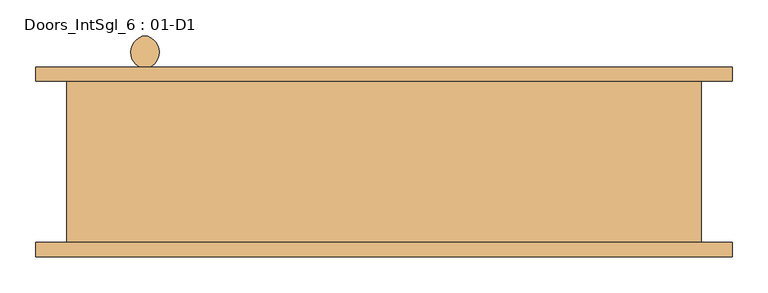
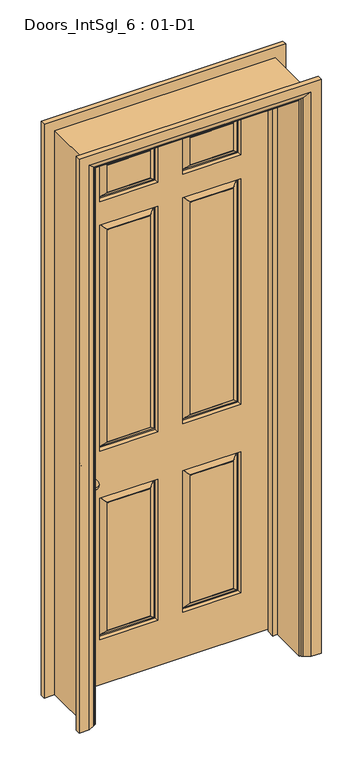
"""IFC4 building model written with IfcOpenShell, lengths in millimetres: door geometry, Doors_IntSgl_6 : 01-D1."""

from ifc_helpers import new_model, si_unit, point, frame, origin, place, context, project, spatial, polyline, circle_curve, ellipse_curve, trimmed, outline, extrude, faceted_brep, source, transform, mapped, element, save
from ifc_brep_helpers import plane_surface, cylinder_surface, revolved_surface, advanced_brep


def doors_intsgl_6_01_d1_adb953bf(model_context):
    return source(origin(), model_context, "Body", "SolidModel", [
        advanced_brep(
        [(-328.0, 55.5, 900.0), (-333.0, 11.062589, 900.0), (-338.0, 55.5, 900.0), (-338.0, 70.5, 900.0), (-328.0, 70.5, 900.0), (-353.0, 74.5, 900.0), (-313.0, 74.5, 900.0), (-353.0, 70.5, 900.0), (-313.0, 70.5, 900.0)],
        [
            (0, 1, circle_curve(frame((-336.1884862, 33.9213505, 900.0), z_axis=(0.0, 0.0, -1.0), x_axis=(0.0, 1.0, 0.0)), 23.0800654)),
            (1, 2, circle_curve(frame((-329.8115138, 33.9213505, 900.0), z_axis=(0.0, 0.0, -1.0), x_axis=(0.0, 1.0, 0.0)), 23.0800654)),
            (2, 0, circle_curve(frame((-333.0, 55.5, 900.0), z_axis=(0.0, -1.0, 0.0), x_axis=(-1.0, 0.0, 0.0)), 5.0)),
            (0, 2, circle_curve(frame((-333.0, 55.5, 900.0), z_axis=(0.0, -1.0, 0.0), x_axis=(-1.0, 0.0, 0.0)), 5.0)),
            (2, 3),
            (3, 4, circle_curve(frame((-333.0, 70.5, 900.0), z_axis=(0.0, -1.0, 0.0), x_axis=(-1.0, 0.0, 0.0)), 5.0)),
            (4, 0),
            (4, 3, circle_curve(frame((-333.0, 70.5, 900.0), z_axis=(0.0, -1.0, 0.0), x_axis=(-1.0, 0.0, 0.0)), 5.0)),
            (5, 6, circle_curve(frame((-333.0, 74.5, 900.0), z_axis=(0.0, 1.0, 0.0), x_axis=(1.0, 0.0, 0.0)), 20.0)),
            (6, 5, circle_curve(frame((-333.0, 74.5, 900.0), z_axis=(0.0, 1.0, 0.0), x_axis=(1.0, 0.0, 0.0)), 20.0)),
            (7, 8, circle_curve(frame((-333.0, 70.5, 900.0), z_axis=(0.0, -1.0, 0.0), x_axis=(1.0, 0.0, 0.0)), 20.0)),
            (8, 7, circle_curve(frame((-333.0, 70.5, 900.0), z_axis=(0.0, -1.0, 0.0), x_axis=(1.0, 0.0, 0.0)), 20.0)),
            (6, 8),
            (7, 5),
        ],
        [
            revolved_surface(trimmed(ellipse_curve(frame((-329.8115138, 33.9213505, 900.0), z_axis=(0.0, 0.0, -1.0), x_axis=(0.0, 1.0, 0.0)), 23.0800654, 23.0800654), [point((-333.0, 11.062589, 900.0))], [point((-338.0, 55.5, 900.0))], True, "CARTESIAN"), (-333.0, 70.5, 900.0), (0.0, 1.0, 0.0)),
            cylinder_surface(frame((-333.0, 70.5, 900.0), z_axis=(0.0, 1.0, 0.0), x_axis=(-1.0, 0.0, 0.0)), 5.0),
            plane_surface(frame((-313.0, 74.5, 900.0), z_axis=(0.0, 1.0, 0.0), x_axis=(0.0, 0.0, 1.0))),
            plane_surface(frame((-313.0, 70.5, 900.0), z_axis=(0.0, -1.0, 0.0), x_axis=(0.0, 0.0, -1.0))),
            cylinder_surface(frame((-333.0, 70.5, 900.0), z_axis=(0.0, 1.0, 0.0), x_axis=(1.0, 0.0, 0.0)), 20.0),
        ],
        [
            (0, [[1, 2, 3]]),
            (0, [[-1, 4, -2]]),
            (1, [[5, 6, 7, -3]]),
            (1, [[-7, 8, -5, -4]]),
            (2, [[9, 10]]),
            (3, [[11, 12], [-8, -6]]),
            (4, [[13, -11, 14, -10]]),
            (4, [[-14, -12, -13, -9]]),
        ],
    ),
        advanced_brep(
        [(-328.0, 131.5, 900.0), (-338.0, 131.5, 900.0), (-333.0, 175.937411, 900.0), (-328.0, 116.5, 900.0), (-338.0, 116.5, 900.0), (-353.0, 112.5, 900.0), (-313.0, 112.5, 900.0), (-353.0, 116.5, 900.0), (-313.0, 116.5, 900.0)],
        [
            (0, 1, circle_curve(frame((-333.0, 131.5, 900.0), z_axis=(0.0, 1.0, 0.0), x_axis=(-1.0, 0.0, 0.0)), 5.0)),
            (1, 2, circle_curve(frame((-329.8115138, 153.0786495, 900.0), z_axis=(0.0, 0.0, -1.0), x_axis=(0.0, -1.0, 0.0)), 23.0800654)),
            (2, 0, circle_curve(frame((-336.1884862, 153.0786495, 900.0), z_axis=(0.0, 0.0, -1.0), x_axis=(0.0, -1.0, 0.0)), 23.0800654)),
            (1, 0, circle_curve(frame((-333.0, 131.5, 900.0), z_axis=(0.0, 1.0, 0.0), x_axis=(-1.0, 0.0, 0.0)), 5.0)),
            (0, 3),
            (3, 4, circle_curve(frame((-333.0, 116.5, 900.0), z_axis=(0.0, 1.0, 0.0), x_axis=(-1.0, 0.0, 0.0)), 5.0)),
            (4, 1),
            (4, 3, circle_curve(frame((-333.0, 116.5, 900.0), z_axis=(0.0, 1.0, 0.0), x_axis=(-1.0, 0.0, 0.0)), 5.0)),
            (5, 6, circle_curve(frame((-333.0, 112.5, 900.0), z_axis=(0.0, -1.0, 0.0), x_axis=(1.0, 0.0, 0.0)), 20.0)),
            (6, 5, circle_curve(frame((-333.0, 112.5, 900.0), z_axis=(0.0, -1.0, 0.0), x_axis=(1.0, 0.0, 0.0)), 20.0)),
            (7, 8, circle_curve(frame((-333.0, 116.5, 900.0), z_axis=(0.0, 1.0, 0.0), x_axis=(1.0, 0.0, 0.0)), 20.0)),
            (8, 7, circle_curve(frame((-333.0, 116.5, 900.0), z_axis=(0.0, 1.0, 0.0), x_axis=(1.0, 0.0, 0.0)), 20.0)),
            (5, 7),
            (8, 6),
        ],
        [
            revolved_surface(trimmed(ellipse_curve(frame((-329.8115138, 153.0786495, 900.0), z_axis=(0.0, 0.0, 1.0), x_axis=(0.0, -1.0, 0.0)), 23.0800654, 23.0800654), [point((-333.0, 175.937411, 900.0))], [point((-338.0, 131.5, 900.0))], True, "CARTESIAN"), (-333.0, 116.5, 900.0), (0.0, -1.0, 0.0)),
            cylinder_surface(frame((-333.0, 116.5, 900.0), z_axis=(0.0, -1.0, 0.0), x_axis=(-1.0, 0.0, 0.0)), 5.0),
            plane_surface(frame((-313.0, 112.5, 900.0), z_axis=(0.0, -1.0, 0.0), x_axis=(0.0, 0.0, 1.0))),
            plane_surface(frame((-313.0, 116.5, 900.0), z_axis=(0.0, 1.0, 0.0), x_axis=(0.0, 0.0, -1.0))),
            cylinder_surface(frame((-333.0, 116.5, 900.0), z_axis=(0.0, -1.0, 0.0), x_axis=(1.0, 0.0, 0.0)), 20.0),
        ],
        [
            (0, [[1, 2, 3]]),
            (0, [[-2, 4, -3]]),
            (1, [[-1, 5, 6, 7]]),
            (1, [[-4, -7, 8, -5]]),
            (2, [[9, 10]]),
            (3, [[11, 12], [-6, -8]]),
            (4, [[-9, 13, -12, 14]]),
            (4, [[-10, -14, -11, -13]]),
        ],
    ),
        faceted_brep([(-408.0, 74.5, 2358.0), (-408.0, 74.5, 8.0), (408.0, 74.5, 8.0), (408.0, 74.5, 2358.0), (-50.0, 74.5, 800.0), (-50.0, 74.5, 200.0), (-283.0, 74.5, 200.0), (-283.0, 74.5, 800.0), (283.0, 74.5, 800.0), (283.0, 74.5, 200.0), (50.0, 74.5, 200.0), (50.0, 74.5, 800.0), (-50.0, 74.5, 1958.0), (-50.0, 74.5, 1000.0), (-283.0, 74.5, 1000.0), (-283.0, 74.5, 1958.0), (283.0, 74.5, 1958.0), (283.0, 74.5, 1000.0), (50.0, 74.5, 1000.0), (50.0, 74.5, 1958.0), (-50.0, 74.5, 2233.0), (-50.0, 74.5, 2058.0), (-283.0, 74.5, 2058.0), (-283.0, 74.5, 2233.0), (283.0, 74.5, 2233.0), (283.0, 74.5, 2058.0), (50.0, 74.5, 2058.0), (50.0, 74.5, 2233.0), (-80.0, 74.5, 230.0), (-80.0, 74.5, 770.0), (-253.0, 74.5, 770.0), (-253.0, 74.5, 230.0), (253.0, 74.5, 230.0), (253.0, 74.5, 770.0), (80.0, 74.5, 770.0), (80.0, 74.5, 230.0), (-80.0, 74.5, 1030.0), (-80.0, 74.5, 1928.0), (-253.0, 74.5, 1928.0), (-253.0, 74.5, 1030.0), (253.0, 74.5, 1030.0), (253.0, 74.5, 1928.0), (80.0, 74.5, 1928.0), (80.0, 74.5, 1030.0), (-80.0, 74.5, 2088.0), (-80.0, 74.5, 2203.0), (-253.0, 74.5, 2203.0), (-253.0, 74.5, 2088.0), (253.0, 74.5, 2088.0), (253.0, 74.5, 2203.0), (80.0, 74.5, 2203.0), (80.0, 74.5, 2088.0), (-408.0, 112.5, 2358.0), (408.0, 112.5, 2358.0), (408.0, 112.5, 8.0), (-408.0, 112.5, 8.0), (50.0, 112.5, 800.0), (50.0, 112.5, 200.0), (283.0, 112.5, 200.0), (283.0, 112.5, 800.0), (-283.0, 112.5, 800.0), (-283.0, 112.5, 200.0), (-50.0, 112.5, 200.0), (-50.0, 112.5, 800.0), (50.0, 112.5, 1958.0), (50.0, 112.5, 1000.0), (283.0, 112.5, 1000.0), (283.0, 112.5, 1958.0), (-283.0, 112.5, 1958.0), (-283.0, 112.5, 1000.0), (-50.0, 112.5, 1000.0), (-50.0, 112.5, 1958.0), (50.0, 112.5, 2233.0), (50.0, 112.5, 2058.0), (283.0, 112.5, 2058.0), (283.0, 112.5, 2233.0), (-283.0, 112.5, 2233.0), (-283.0, 112.5, 2058.0), (-50.0, 112.5, 2058.0), (-50.0, 112.5, 2233.0), (80.0, 112.5, 230.0), (80.0, 112.5, 770.0), (253.0, 112.5, 770.0), (253.0, 112.5, 230.0), (-253.0, 112.5, 230.0), (-253.0, 112.5, 770.0), (-80.0, 112.5, 770.0), (-80.0, 112.5, 230.0), (80.0, 112.5, 1030.0), (80.0, 112.5, 1928.0), (253.0, 112.5, 1928.0), (253.0, 112.5, 1030.0), (-253.0, 112.5, 1030.0), (-253.0, 112.5, 1928.0), (-80.0, 112.5, 1928.0), (-80.0, 112.5, 1030.0), (80.0, 112.5, 2088.0), (80.0, 112.5, 2203.0), (253.0, 112.5, 2203.0), (253.0, 112.5, 2088.0), (-253.0, 112.5, 2088.0), (-253.0, 112.5, 2203.0), (-80.0, 112.5, 2203.0), (-80.0, 112.5, 2088.0), (80.0, 111.5, 230.0), (80.0, 111.5, 770.0), (58.0, 97.5, 208.0), (58.0, 97.5, 792.0), (78.0, 111.5, 772.0), (78.0, 111.5, 228.0), (53.0, 97.5, 797.0), (53.0, 97.5, 203.0), (253.0, 111.5, 770.0), (275.0, 97.5, 792.0), (255.0, 111.5, 772.0), (280.0, 97.5, 797.0), (253.0, 111.5, 230.0), (275.0, 97.5, 208.0), (255.0, 111.5, 228.0), (280.0, 97.5, 203.0), (-253.0, 111.5, 230.0), (-253.0, 111.5, 770.0), (-275.0, 97.5, 208.0), (-275.0, 97.5, 792.0), (-255.0, 111.5, 772.0), (-255.0, 111.5, 228.0), (-280.0, 97.5, 797.0), (-280.0, 97.5, 203.0), (-80.0, 111.5, 770.0), (-58.0, 97.5, 792.0), (-78.0, 111.5, 772.0), (-53.0, 97.5, 797.0), (-80.0, 111.5, 230.0), (-58.0, 97.5, 208.0), (-78.0, 111.5, 228.0), (-53.0, 97.5, 203.0), (80.0, 111.5, 1030.0), (80.0, 111.5, 1928.0), (58.0, 97.5, 1008.0), (58.0, 97.5, 1950.0), (78.0, 111.5, 1930.0), (78.0, 111.5, 1028.0), (53.0, 97.5, 1955.0), (53.0, 97.5, 1003.0), (253.0, 111.5, 1928.0), (275.0, 97.5, 1950.0), (255.0, 111.5, 1930.0), (280.0, 97.5, 1955.0), (253.0, 111.5, 1030.0), (275.0, 97.5, 1008.0), (255.0, 111.5, 1028.0), (280.0, 97.5, 1003.0), (-253.0, 111.5, 1030.0), (-253.0, 111.5, 1928.0), (-275.0, 97.5, 1008.0), (-275.0, 97.5, 1950.0), (-255.0, 111.5, 1930.0), (-255.0, 111.5, 1028.0), (-280.0, 97.5, 1955.0), (-280.0, 97.5, 1003.0), (-80.0, 111.5, 1928.0), (-58.0, 97.5, 1950.0), (-78.0, 111.5, 1930.0), (-53.0, 97.5, 1955.0), (-80.0, 111.5, 1030.0), (-58.0, 97.5, 1008.0), (-78.0, 111.5, 1028.0), (-53.0, 97.5, 1003.0), (80.0, 111.5, 2088.0), (80.0, 111.5, 2203.0), (58.0, 97.5, 2066.0), (58.0, 97.5, 2225.0), (78.0, 111.5, 2205.0), (78.0, 111.5, 2086.0), (53.0, 97.5, 2230.0), (53.0, 97.5, 2061.0), (253.0, 111.5, 2203.0), (275.0, 97.5, 2225.0), (255.0, 111.5, 2205.0), (280.0, 97.5, 2230.0), (253.0, 111.5, 2088.0), (275.0, 97.5, 2066.0), (255.0, 111.5, 2086.0), (280.0, 97.5, 2061.0), (-253.0, 111.5, 2088.0), (-253.0, 111.5, 2203.0), (-275.0, 97.5, 2066.0), (-275.0, 97.5, 2225.0), (-255.0, 111.5, 2205.0), (-255.0, 111.5, 2086.0), (-280.0, 97.5, 2230.0), (-280.0, 97.5, 2061.0), (-80.0, 111.5, 2203.0), (-58.0, 97.5, 2225.0), (-78.0, 111.5, 2205.0), (-53.0, 97.5, 2230.0), (-80.0, 111.5, 2088.0), (-58.0, 97.5, 2066.0), (-78.0, 111.5, 2086.0), (-53.0, 97.5, 2061.0), (-80.0, 75.5, 230.0), (-80.0, 75.5, 770.0), (-58.0, 89.5, 208.0), (-58.0, 89.5, 792.0), (-78.0, 75.5, 772.0), (-78.0, 75.5, 228.0), (-53.0, 89.5, 797.0), (-53.0, 89.5, 203.0), (-253.0, 75.5, 770.0), (-275.0, 89.5, 792.0), (-255.0, 75.5, 772.0), (-280.0, 89.5, 797.0), (-253.0, 75.5, 230.0), (-275.0, 89.5, 208.0), (-255.0, 75.5, 228.0), (-280.0, 89.5, 203.0), (253.0, 75.5, 230.0), (253.0, 75.5, 770.0), (275.0, 89.5, 208.0), (275.0, 89.5, 792.0), (255.0, 75.5, 772.0), (255.0, 75.5, 228.0), (280.0, 89.5, 797.0), (280.0, 89.5, 203.0), (80.0, 75.5, 770.0), (58.0, 89.5, 792.0), (78.0, 75.5, 772.0), (53.0, 89.5, 797.0), (80.0, 75.5, 230.0), (58.0, 89.5, 208.0), (78.0, 75.5, 228.0), (53.0, 89.5, 203.0), (-80.0, 75.5, 1030.0), (-80.0, 75.5, 1928.0), (-58.0, 89.5, 1008.0), (-58.0, 89.5, 1950.0), (-78.0, 75.5, 1930.0), (-78.0, 75.5, 1028.0), (-53.0, 89.5, 1955.0), (-53.0, 89.5, 1003.0), (-253.0, 75.5, 1928.0), (-275.0, 89.5, 1950.0), (-255.0, 75.5, 1930.0), (-280.0, 89.5, 1955.0), (-253.0, 75.5, 1030.0), (-275.0, 89.5, 1008.0), (-255.0, 75.5, 1028.0), (-280.0, 89.5, 1003.0), (253.0, 75.5, 1030.0), (253.0, 75.5, 1928.0), (275.0, 89.5, 1008.0), (275.0, 89.5, 1950.0), (255.0, 75.5, 1930.0), (255.0, 75.5, 1028.0), (280.0, 89.5, 1955.0), (280.0, 89.5, 1003.0), (80.0, 75.5, 1928.0), (58.0, 89.5, 1950.0), (78.0, 75.5, 1930.0), (53.0, 89.5, 1955.0), (80.0, 75.5, 1030.0), (58.0, 89.5, 1008.0), (78.0, 75.5, 1028.0), (53.0, 89.5, 1003.0), (-80.0, 75.5, 2088.0), (-80.0, 75.5, 2203.0), (-58.0, 89.5, 2066.0), (-58.0, 89.5, 2225.0), (-78.0, 75.5, 2205.0), (-78.0, 75.5, 2086.0), (-53.0, 89.5, 2230.0), (-53.0, 89.5, 2061.0), (-253.0, 75.5, 2203.0), (-275.0, 89.5, 2225.0), (-255.0, 75.5, 2205.0), (-280.0, 89.5, 2230.0), (-253.0, 75.5, 2088.0), (-275.0, 89.5, 2066.0), (-255.0, 75.5, 2086.0), (-280.0, 89.5, 2061.0), (253.0, 75.5, 2088.0), (253.0, 75.5, 2203.0), (275.0, 89.5, 2066.0), (275.0, 89.5, 2225.0), (255.0, 75.5, 2205.0), (255.0, 75.5, 2086.0), (280.0, 89.5, 2230.0), (280.0, 89.5, 2061.0), (80.0, 75.5, 2203.0), (58.0, 89.5, 2225.0), (78.0, 75.5, 2205.0), (53.0, 89.5, 2230.0), (80.0, 75.5, 2088.0), (58.0, 89.5, 2066.0), (78.0, 75.5, 2086.0), (53.0, 89.5, 2061.0)], [[[0, 1, 2, 3], [4, 5, 6, 7], [8, 9, 10, 11], [12, 13, 14, 15], [16, 17, 18, 19], [20, 21, 22, 23], [24, 25, 26, 27]], [[28, 29, 30, 31]], [[32, 33, 34, 35]], [[36, 37, 38, 39]], [[40, 41, 42, 43]], [[44, 45, 46, 47]], [[48, 49, 50, 51]], [[52, 53, 54, 55], [56, 57, 58, 59], [60, 61, 62, 63], [64, 65, 66, 67], [68, 69, 70, 71], [72, 73, 74, 75], [76, 77, 78, 79]], [[80, 81, 82, 83]], [[84, 85, 86, 87]], [[88, 89, 90, 91]], [[92, 93, 94, 95]], [[96, 97, 98, 99]], [[100, 101, 102, 103]], [[1, 0, 52, 55]], [[2, 1, 55, 54]], [[3, 2, 54, 53]], [[0, 3, 53, 52]], [[104, 105, 81, 80]], [[106, 107, 108, 109]], [[56, 110, 111, 57]], [[81, 105, 112, 82]], [[108, 107, 113, 114]], [[110, 56, 59, 115]], [[82, 112, 116, 83]], [[114, 113, 117, 118]], [[115, 59, 58, 119]], [[104, 80, 83, 116]], [[109, 108, 114, 118], [105, 104, 116, 112]], [[106, 109, 118, 117]], [[111, 110, 115, 119], [107, 106, 117, 113]], [[57, 111, 119, 58]], [[120, 121, 85, 84]], [[122, 123, 124, 125]], [[60, 126, 127, 61]], [[85, 121, 128, 86]], [[124, 123, 129, 130]], [[126, 60, 63, 131]], [[86, 128, 132, 87]], [[130, 129, 133, 134]], [[131, 63, 62, 135]], [[120, 84, 87, 132]], [[125, 124, 130, 134], [121, 120, 132, 128]], [[122, 125, 134, 133]], [[127, 126, 131, 135], [123, 122, 133, 129]], [[61, 127, 135, 62]], [[136, 137, 89, 88]], [[138, 139, 140, 141]], [[64, 142, 143, 65]], [[89, 137, 144, 90]], [[140, 139, 145, 146]], [[142, 64, 67, 147]], [[90, 144, 148, 91]], [[146, 145, 149, 150]], [[147, 67, 66, 151]], [[136, 88, 91, 148]], [[141, 140, 146, 150], [137, 136, 148, 144]], [[138, 141, 150, 149]], [[143, 142, 147, 151], [139, 138, 149, 145]], [[65, 143, 151, 66]], [[152, 153, 93, 92]], [[154, 155, 156, 157]], [[68, 158, 159, 69]], [[93, 153, 160, 94]], [[156, 155, 161, 162]], [[158, 68, 71, 163]], [[94, 160, 164, 95]], [[162, 161, 165, 166]], [[163, 71, 70, 167]], [[152, 92, 95, 164]], [[157, 156, 162, 166], [153, 152, 164, 160]], [[154, 157, 166, 165]], [[159, 158, 163, 167], [155, 154, 165, 161]], [[69, 159, 167, 70]], [[168, 169, 97, 96]], [[170, 171, 172, 173]], [[72, 174, 175, 73]], [[97, 169, 176, 98]], [[172, 171, 177, 178]], [[174, 72, 75, 179]], [[98, 176, 180, 99]], [[178, 177, 181, 182]], [[179, 75, 74, 183]], [[168, 96, 99, 180]], [[173, 172, 178, 182], [169, 168, 180, 176]], [[170, 173, 182, 181]], [[175, 174, 179, 183], [171, 170, 181, 177]], [[73, 175, 183, 74]], [[184, 185, 101, 100]], [[186, 187, 188, 189]], [[76, 190, 191, 77]], [[101, 185, 192, 102]], [[188, 187, 193, 194]], [[190, 76, 79, 195]], [[102, 192, 196, 103]], [[194, 193, 197, 198]], [[195, 79, 78, 199]], [[184, 100, 103, 196]], [[189, 188, 194, 198], [185, 184, 196, 192]], [[186, 189, 198, 197]], [[191, 190, 195, 199], [187, 186, 197, 193]], [[77, 191, 199, 78]], [[200, 201, 29, 28]], [[202, 203, 204, 205]], [[4, 206, 207, 5]], [[29, 201, 208, 30]], [[204, 203, 209, 210]], [[206, 4, 7, 211]], [[30, 208, 212, 31]], [[210, 209, 213, 214]], [[211, 7, 6, 215]], [[200, 28, 31, 212]], [[205, 204, 210, 214], [201, 200, 212, 208]], [[202, 205, 214, 213]], [[207, 206, 211, 215], [203, 202, 213, 209]], [[5, 207, 215, 6]], [[216, 217, 33, 32]], [[218, 219, 220, 221]], [[8, 222, 223, 9]], [[33, 217, 224, 34]], [[220, 219, 225, 226]], [[222, 8, 11, 227]], [[34, 224, 228, 35]], [[226, 225, 229, 230]], [[227, 11, 10, 231]], [[216, 32, 35, 228]], [[221, 220, 226, 230], [217, 216, 228, 224]], [[218, 221, 230, 229]], [[223, 222, 227, 231], [219, 218, 229, 225]], [[9, 223, 231, 10]], [[232, 233, 37, 36]], [[234, 235, 236, 237]], [[12, 238, 239, 13]], [[37, 233, 240, 38]], [[236, 235, 241, 242]], [[238, 12, 15, 243]], [[38, 240, 244, 39]], [[242, 241, 245, 246]], [[243, 15, 14, 247]], [[232, 36, 39, 244]], [[237, 236, 242, 246], [233, 232, 244, 240]], [[234, 237, 246, 245]], [[239, 238, 243, 247], [235, 234, 245, 241]], [[13, 239, 247, 14]], [[248, 249, 41, 40]], [[250, 251, 252, 253]], [[16, 254, 255, 17]], [[41, 249, 256, 42]], [[252, 251, 257, 258]], [[254, 16, 19, 259]], [[42, 256, 260, 43]], [[258, 257, 261, 262]], [[259, 19, 18, 263]], [[248, 40, 43, 260]], [[253, 252, 258, 262], [249, 248, 260, 256]], [[250, 253, 262, 261]], [[255, 254, 259, 263], [251, 250, 261, 257]], [[17, 255, 263, 18]], [[264, 265, 45, 44]], [[266, 267, 268, 269]], [[20, 270, 271, 21]], [[45, 265, 272, 46]], [[268, 267, 273, 274]], [[270, 20, 23, 275]], [[46, 272, 276, 47]], [[274, 273, 277, 278]], [[275, 23, 22, 279]], [[264, 44, 47, 276]], [[269, 268, 274, 278], [265, 264, 276, 272]], [[266, 269, 278, 277]], [[271, 270, 275, 279], [267, 266, 277, 273]], [[21, 271, 279, 22]], [[280, 281, 49, 48]], [[282, 283, 284, 285]], [[24, 286, 287, 25]], [[49, 281, 288, 50]], [[284, 283, 289, 290]], [[286, 24, 27, 291]], [[50, 288, 292, 51]], [[290, 289, 293, 294]], [[291, 27, 26, 295]], [[280, 48, 51, 292]], [[285, 284, 290, 294], [281, 280, 292, 288]], [[282, 285, 294, 293]], [[287, 286, 291, 295], [283, 282, 293, 289]], [[25, 287, 295, 26]]]),
        faceted_brep([(-410.0, 112.5, 0.0), (-410.0, -112.5, 0.0), (-442.0, -112.5, 0.0), (-442.0, 112.5, 0.0), (-410.0, 112.5, 2360.0), (-410.0, -112.5, 2360.0), (-442.0, -112.5, 2392.0), (-442.0, 112.5, 2392.0), (410.0, 112.5, 0.0), (442.0, 112.5, 0.0), (442.0, -112.5, 0.0), (410.0, -112.5, 0.0), (410.0, 112.5, 2360.0), (442.0, 112.5, 2392.0), (442.0, -112.5, 2392.0), (410.0, -112.5, 2360.0)], [[[0, 1, 2, 3]], [[1, 0, 4, 5]], [[2, 1, 5, 6]], [[3, 2, 6, 7]], [[0, 3, 7, 4]], [[8, 9, 10, 11]], [[12, 13, 9, 8]], [[13, 14, 10, 9]], [[14, 15, 11, 10]], [[15, 12, 8, 11]], [[5, 4, 12, 15]], [[6, 5, 15, 14]], [[7, 6, 14, 13]], [[4, 7, 13, 12]]]),
        extrude(outline(polyline([(0.0, -410.0), (0.0, -391.0), (2341.0, -391.0), (2341.0, 391.0), (0.0, 391.0), (0.0, 410.0), (2360.0, 410.0), (2360.0, -410.0), (0.0, -410.0)])), frame((0.0, 40.5, 0.0), z_axis=(0.0, 1.0, 0.0), x_axis=(0.0, 0.0, 1.0)), (0.0, 0.0, 1.0), 32.0),
        advanced_brep(
        [(-485.0, -132.5, 0.0), (-485.0, -112.5, 0.0), (-415.0, -112.5, 0.0), (-419.0, -118.5, 0.0), (-445.0, -132.5, 0.0), (-485.0, -132.5, 2435.0), (-485.0, -112.5, 2435.0), (485.0, -112.5, 2435.0), (485.0, -112.5, 0.0), (415.0, -112.5, 0.0), (415.0, -112.5, 2365.0), (-415.0, -112.5, 2365.0), (-419.0, -118.5, 2369.0), (-445.0, -132.5, 2395.0), (445.0, -132.5, 2395.0), (445.0, -132.5, 0.0), (485.0, -132.5, 0.0), (485.0, -132.5, 2435.0), (419.0, -118.5, 0.0), (419.0, -118.5, 2369.0)],
        [
            (0, 1),
            (1, 2),
            (2, 3, circle_curve(frame((-423.0, -111.5, 0.0), z_axis=(0.0, 0.0, -1.0), x_axis=(-1.0, 0.0, 0.0)), 8.0622577)),
            (3, 4),
            (4, 0),
            (0, 5),
            (5, 6),
            (6, 1),
            (6, 7),
            (7, 8),
            (8, 9),
            (9, 10),
            (10, 11),
            (11, 2),
            (11, 12, ellipse_curve(frame((-423.0, -111.5, 2373.0), z_axis=(-0.7071067811865475, 0.0, -0.7071067811865475), x_axis=(0.7071067811865474, 0.0, -0.7071067811865476)), 11.4017543, 8.0622577)),
            (12, 3),
            (12, 13),
            (13, 4),
            (13, 14),
            (14, 15),
            (15, 16),
            (16, 17),
            (17, 5),
            (7, 17),
            (16, 8),
            (15, 18),
            (18, 9, circle_curve(frame((423.0, -111.5, 0.0), z_axis=(0.0, 0.0, -1.0), x_axis=(1.0, 0.0, 0.0)), 8.0622577)),
            (19, 10, ellipse_curve(frame((423.0, -111.5, 2373.0), z_axis=(0.7071067811865475, 0.0, -0.7071067811865475), x_axis=(0.7071067811865474, 0.0, 0.7071067811865476)), 11.4017543, 8.0622577)),
            (18, 19),
            (14, 19),
            (19, 12),
        ],
        [
            plane_surface(frame((-415.0, -112.5, 0.0), z_axis=(0.0, 0.0, -1.0), x_axis=(0.0, -1.0, 0.0))),
            plane_surface(frame((-485.0, -132.5, 0.0), z_axis=(-1.0, 0.0, 0.0), x_axis=(0.0, 0.0, 1.0))),
            plane_surface(frame((-485.0, -112.5, 0.0), z_axis=(0.0, 1.0, 0.0), x_axis=(0.0, 0.0, 1.0))),
            cylinder_surface(frame((-423.0, -111.5, 0.0), z_axis=(0.0, 0.0, -1.0), x_axis=(-1.0, 0.0, 0.0)), 8.0622577),
            plane_surface(frame((-419.0, -118.5, 0.0), z_axis=(0.4740998230350183, -0.8804710999221749, 0.0), x_axis=(0.0, 0.0, 1.0))),
            plane_surface(frame((-445.0, -132.5, 0.0), z_axis=(0.0, -1.0, 0.0), x_axis=(0.0, 0.0, 1.0))),
            plane_surface(frame((485.0, -132.5, 2435.0), z_axis=(1.0, 0.0, 0.0), x_axis=(0.0, 0.0, -1.0))),
            plane_surface(frame((415.0, -112.5, 0.0), z_axis=(0.0, 0.0, -1.0), x_axis=(0.0, -1.0, 0.0))),
            cylinder_surface(frame((423.0, -111.5, 2365.0), z_axis=(0.0, 0.0, 1.0), x_axis=(1.0, 0.0, 0.0)), 8.0622577),
            plane_surface(frame((419.0, -118.5, 2369.0), z_axis=(-0.4740998230350183, -0.8804710999221749, 0.0), x_axis=(0.0, 0.0, -1.0))),
            plane_surface(frame((-485.0, -132.5, 2435.0), z_axis=(0.0, 0.0, 1.0), x_axis=(1.0, 0.0, 0.0))),
            cylinder_surface(frame((-415.0, -111.5, 2373.0), z_axis=(-1.0, 0.0, 0.0), x_axis=(0.0, 0.0, 1.0)), 8.0622577),
            plane_surface(frame((-419.0, -118.5, 2369.0), z_axis=(0.0, -0.8804710999221749, -0.4740998230350183), x_axis=(1.0, 0.0, 0.0))),
        ],
        [
            (0, [[1, 2, 3, 4, 5]]),
            (1, [[-1, 6, 7, 8]]),
            (2, [[-2, -8, 9, 10, 11, 12, 13, 14]]),
            (3, [[-3, -14, 15, 16]]),
            (4, [[-4, -16, 17, 18]]),
            (5, [[-5, -18, 19, 20, 21, 22, 23, -6]]),
            (6, [[24, -22, 25, -10]]),
            (7, [[-21, 26, 27, -11, -25]]),
            (8, [[28, -12, -27, 29]]),
            (9, [[30, -29, -26, -20]]),
            (10, [[-7, -23, -24, -9]]),
            (11, [[-15, -13, -28, 31]]),
            (12, [[-17, -31, -30, -19]]),
        ],
    ),
        advanced_brep(
        [(485.0, 132.5, 0.0), (485.0, 112.5, 0.0), (415.0, 112.5, 0.0), (419.0, 118.5, 0.0), (445.0, 132.5, 0.0), (485.0, 132.5, 2435.0), (485.0, 112.5, 2435.0), (-485.0, 112.5, 2435.0), (-485.0, 112.5, 0.0), (-415.0, 112.5, 0.0), (-415.0, 112.5, 2365.0), (415.0, 112.5, 2365.0), (419.0, 118.5, 2369.0), (445.0, 132.5, 2395.0), (-445.0, 132.5, 2395.0), (-445.0, 132.5, 0.0), (-485.0, 132.5, 0.0), (-485.0, 132.5, 2435.0), (-419.0, 118.5, 0.0), (-419.0, 118.5, 2369.0)],
        [
            (0, 1),
            (1, 2),
            (2, 3, circle_curve(frame((423.0, 111.5, 0.0), z_axis=(0.0, 0.0, -1.0), x_axis=(1.0, 0.0, 0.0)), 8.0622577)),
            (3, 4),
            (4, 0),
            (0, 5),
            (5, 6),
            (6, 1),
            (6, 7),
            (7, 8),
            (8, 9),
            (9, 10),
            (10, 11),
            (11, 2),
            (11, 12, ellipse_curve(frame((423.0, 111.5, 2373.0), z_axis=(0.7071067811865475, 0.0, -0.7071067811865475), x_axis=(-0.7071067811865474, 0.0, -0.7071067811865476)), 11.4017543, 8.0622577)),
            (12, 3),
            (12, 13),
            (13, 4),
            (13, 14),
            (14, 15),
            (15, 16),
            (16, 17),
            (17, 5),
            (7, 17),
            (16, 8),
            (15, 18),
            (18, 9, circle_curve(frame((-423.0, 111.5, 0.0), z_axis=(0.0, 0.0, -1.0), x_axis=(-1.0, 0.0, 0.0)), 8.0622577)),
            (19, 10, ellipse_curve(frame((-423.0, 111.5, 2373.0), z_axis=(-0.7071067811865475, 0.0, -0.7071067811865475), x_axis=(-0.7071067811865474, 0.0, 0.7071067811865476)), 11.4017543, 8.0622577)),
            (18, 19),
            (14, 19),
            (19, 12),
        ],
        [
            plane_surface(frame((415.0, 112.5, 0.0), z_axis=(0.0, 0.0, -1.0), x_axis=(0.0, 1.0, 0.0))),
            plane_surface(frame((485.0, 132.5, 0.0), z_axis=(1.0, 0.0, 0.0), x_axis=(0.0, 0.0, 1.0))),
            plane_surface(frame((485.0, 112.5, 0.0), z_axis=(0.0, -1.0, 0.0), x_axis=(0.0, 0.0, 1.0))),
            cylinder_surface(frame((423.0, 111.5, 0.0), z_axis=(0.0, 0.0, -1.0), x_axis=(1.0, 0.0, 0.0)), 8.0622577),
            plane_surface(frame((419.0, 118.5, 0.0), z_axis=(-0.4740998230350183, 0.8804710999221749, 0.0), x_axis=(0.0, 0.0, 1.0))),
            plane_surface(frame((445.0, 132.5, 0.0), z_axis=(0.0, 1.0, 0.0), x_axis=(0.0, 0.0, 1.0))),
            plane_surface(frame((-485.0, 132.5, 2435.0), z_axis=(-1.0, 0.0, 0.0), x_axis=(0.0, 0.0, -1.0))),
            plane_surface(frame((-415.0, 112.5, 0.0), z_axis=(0.0, 0.0, -1.0), x_axis=(0.0, 1.0, 0.0))),
            cylinder_surface(frame((-423.0, 111.5, 2365.0), z_axis=(0.0, 0.0, 1.0), x_axis=(-1.0, 0.0, 0.0)), 8.0622577),
            plane_surface(frame((-419.0, 118.5, 2369.0), z_axis=(0.4740998230350183, 0.8804710999221749, 0.0), x_axis=(0.0, 0.0, -1.0))),
            plane_surface(frame((485.0, 132.5, 2435.0), z_axis=(0.0, 0.0, 1.0), x_axis=(-1.0, 0.0, 0.0))),
            cylinder_surface(frame((415.0, 111.5, 2373.0), z_axis=(1.0, 0.0, 0.0), x_axis=(0.0, 0.0, 1.0)), 8.0622577),
            plane_surface(frame((419.0, 118.5, 2369.0), z_axis=(0.0, 0.8804710999221749, -0.4740998230350183), x_axis=(-1.0, 0.0, 0.0))),
        ],
        [
            (0, [[1, 2, 3, 4, 5]]),
            (1, [[-1, 6, 7, 8]]),
            (2, [[-2, -8, 9, 10, 11, 12, 13, 14]]),
            (3, [[-3, -14, 15, 16]]),
            (4, [[-4, -16, 17, 18]]),
            (5, [[-5, -18, 19, 20, 21, 22, 23, -6]]),
            (6, [[24, -22, 25, -10]]),
            (7, [[-21, 26, 27, -11, -25]]),
            (8, [[28, -12, -27, 29]]),
            (9, [[30, -29, -26, -20]]),
            (10, [[-7, -23, -24, -9]]),
            (11, [[-15, -13, -28, 31]]),
            (12, [[-17, -31, -30, -19]]),
        ],
    ),
    ])


if __name__ == "__main__":
    model = new_model("IFC4")
    model_context = context("Model", 3, world=origin())
    ifc_project = project(units=[si_unit("LENGTHUNIT", "METRE", prefix="MILLI")], contexts=[model_context])
    site = spatial("IfcSite", under=ifc_project)
    building = spatial("IfcBuilding", under=site)
    placement = place(None, origin())
    doors_intsgl_6_01_d1_shape = doors_intsgl_6_01_d1_adb953bf(model_context)
    element("IfcDoor", 1, ObjectType="Doors_IntSgl_6 : 01-D1", at=placement, inside=building, context=model_context, shape_type="MappedRepresentation", body=[
        mapped(doors_intsgl_6_01_d1_shape, transform((0.0, 0.0, 0.0), x_axis=(1.0, 0.0, 0.0), y_axis=(0.0, 1.0, 0.0), z_axis=(0.0, 0.0, 1.0))),
    ])
    save(model, "model.ifc")

# Revit data of these elements
# Type "Doors_IntSgl_6 : 01-D1"
#   Type Mark = "49"
#   Type Comments = "Internal Single"
#   Operation = "SingleSwingRight"
#   Construction Type Id = "MDOOR"
#   Manufacturer = "Revit"
#   Keynote = "L20"
#   Description = "Internal Single Door"
#   Analytic Construction = "Metal"
#   UnderCut = 8 mm
#   Tolerance = 2 mm
#   Thickness = 38 mm
#   Structural Tolerance = 8 mm
#   StopDepth = 32 mm
#   Stop Thickness = 19 mm
#   Stile Top Rail = 125 mm
#   Stile Shutting = 125 mm
#   Stile Muntin Rail = 100 mm
#   Stile Lock Rail = 200 mm
#   Stile Intermediate/Frieze = 100 mm
#   Stile Hanging = 125 mm
#   Stile Bottom Rail = 200 mm
#   Rough Width = 900 mm
#   Rough Height = 2400 mm
#   Height to Top Lock Rail = 1000 mm
#   Heat Transfer Coefficient (U) = 3.7021 W/(m²·K)
#   Handle Z Distance = 900 mm
#   Handle X Distance = 75 mm
#   Frame Thickness = 32 mm
#   Door Panel Width = 816 mm
#   Height = 2400 mm
#   Width = 900 mm
#   Door Panel Thickness = 38 mm
#   Door Panel Offset = 0 mm
#   Door Panel Height = 2350 mm
#   Architrave Setback = 5 mm
#   Vis - Ironmongery = yes
#   Define Thermal Properties by = 1
#   Material Ironmongery = Door - Handle
#   Material Frame = Door - Frame/Mullion
#   Material Door = Door - Panel
#   Material Architrave = Door - Architrave
#   Visual Light Transmittance = 0
#   Solar Heat Gain Coefficient = 0
#   Function = (empty or 0)
#   Wall Closure = (empty or 0)
# Element 1 (IfcDoor, "Doors_IntSgl_6 : 01-D1")
#   Materials on its faces: "Door - Panel", "Door - Architrave", "Door - Frame/Mullion", "Door - Handle"
# Materials
#   "Door - Handle": colour RGB 247 247 247, transparency 0
#   "Door - Frame/Mullion": class "Wood", colour RGB 212 179 113, transparency 0
#   "Door - Panel": class "Wood", colour RGB 154 90 5, transparency 0
#   "Door - Architrave": class "Wood", colour RGB 154 90 5, transparency 0
